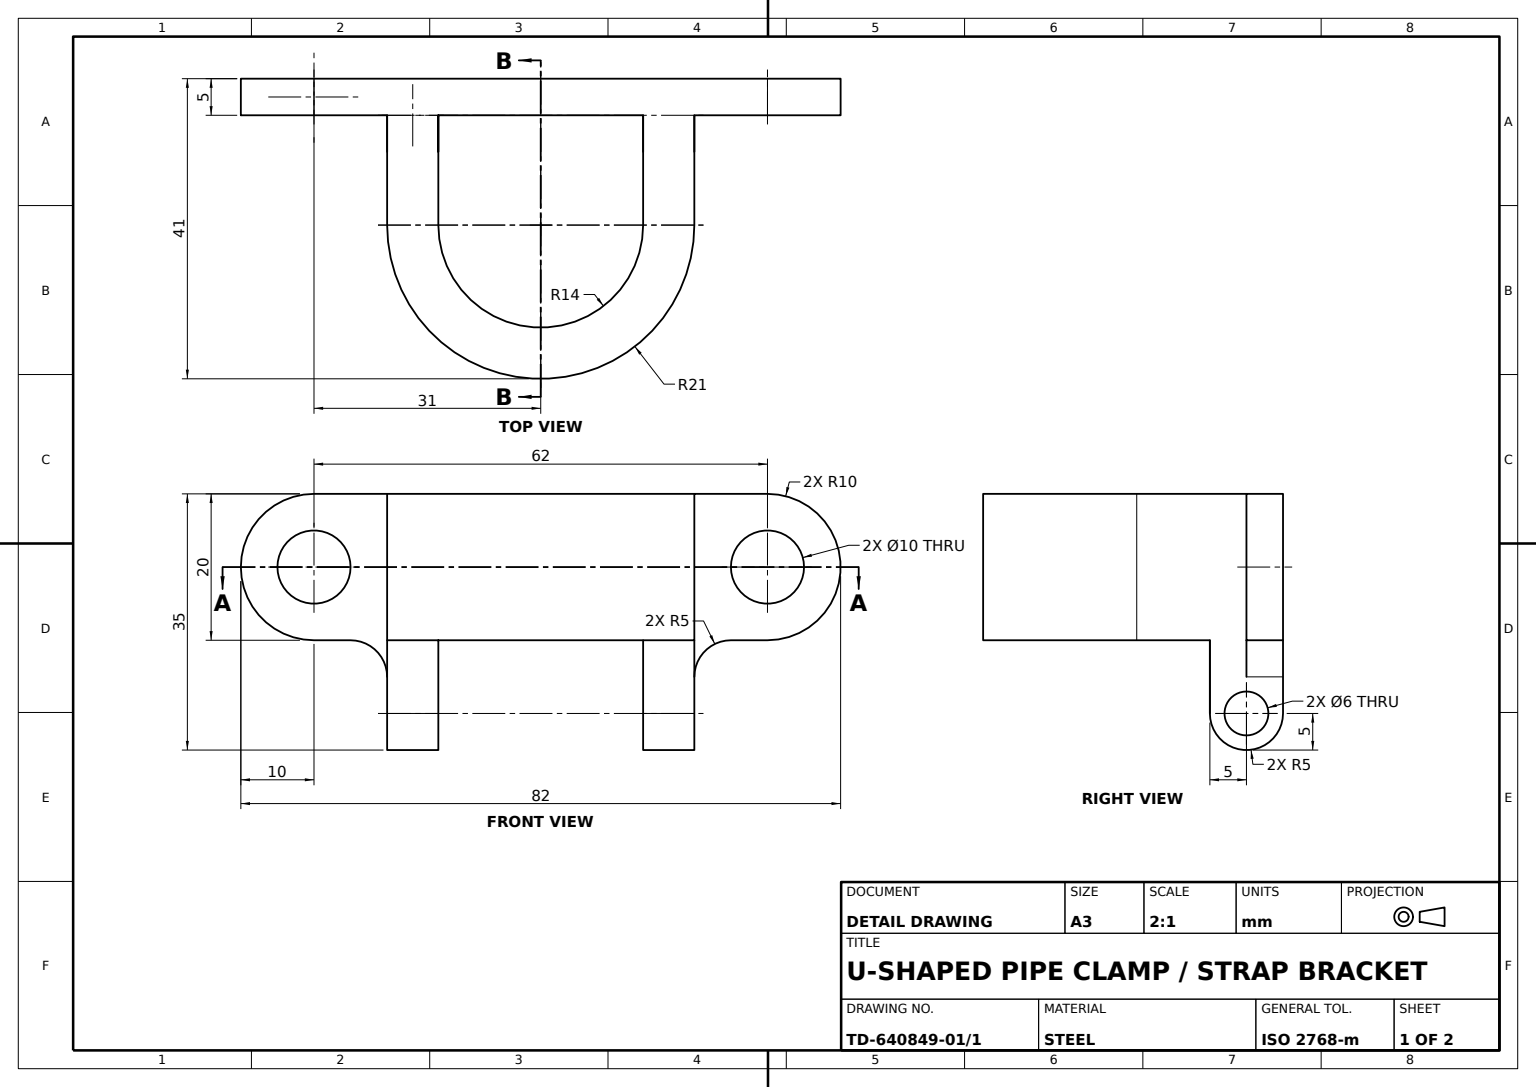
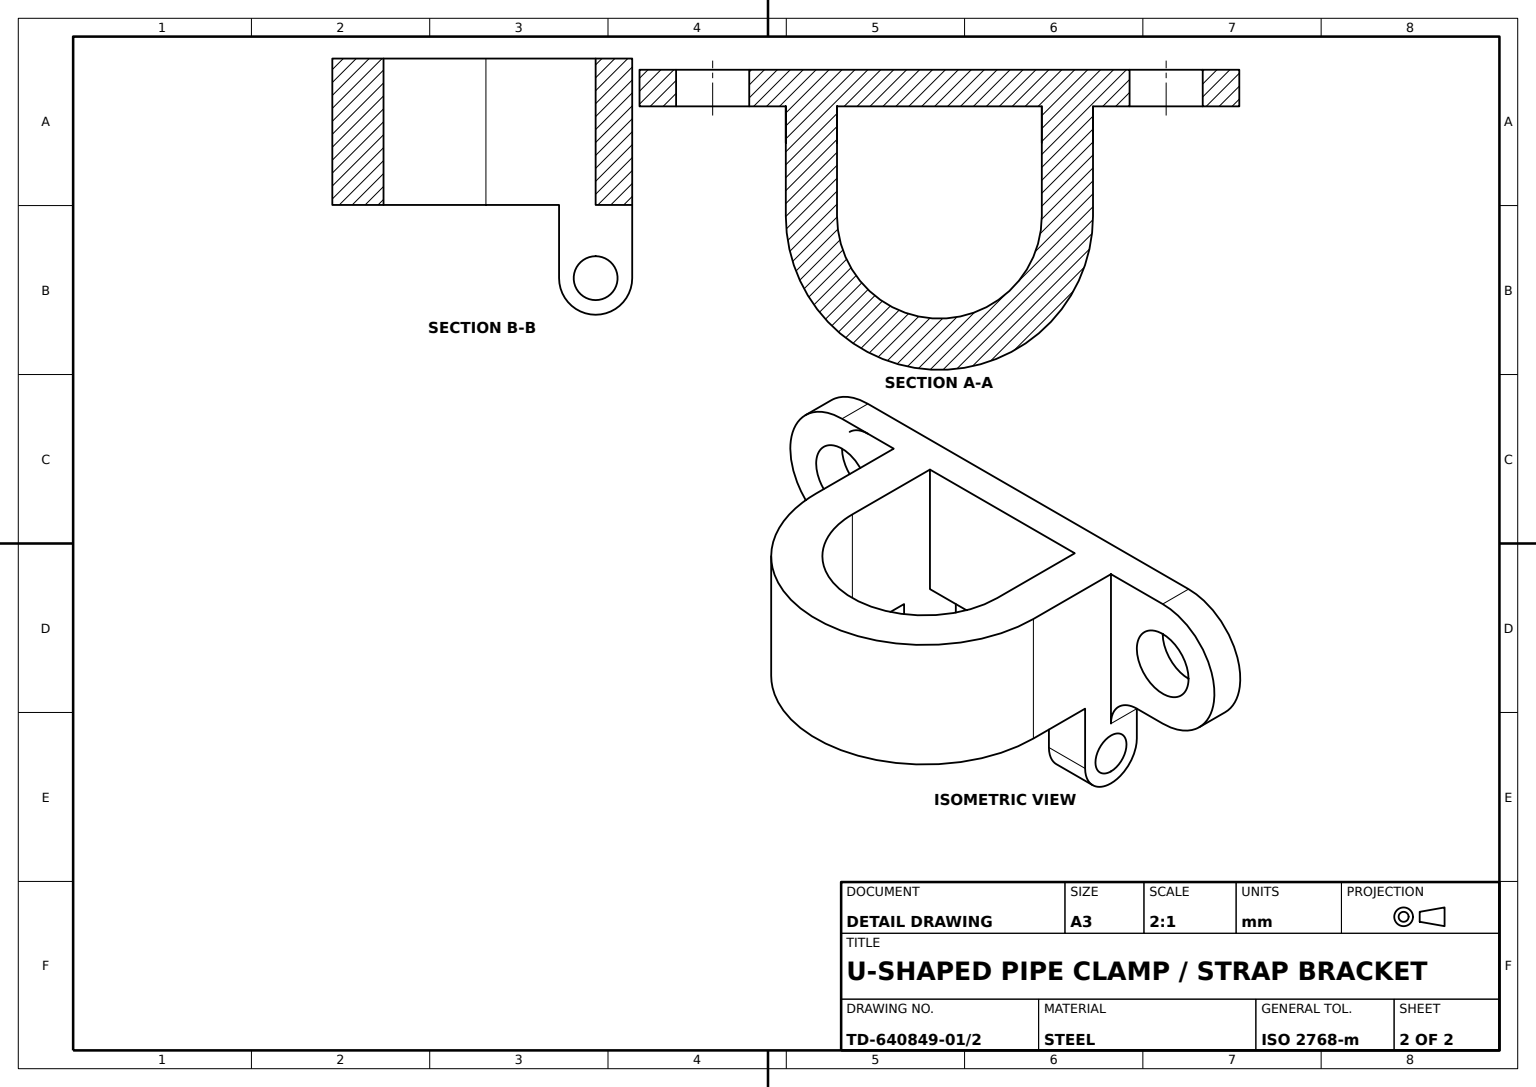
SolidWorks part; units mm, degrees
material "Plain Carbon Steel"
ref_plane "Front Plane" through (0, 0, 0) normal (0, 0, 1) x (1, 0, 0)
ref_plane "Top Plane" through (0, 0, 0) normal (0, 1, 0) x (1, 0, 0)
ref_plane "Right Plane" through (0, 0, 0) normal (1, 0, 0) x (0, 0, -1)
sketch "Base Flange Sketch" plane through (0, 0, 0) normal (0, 0, 1) x (1, 0, 0)
  line L2 (0, 10) -> (62, 10)
  line L4 (62, -10) -> (0, -10)
  line L5 (0, -10) -> (10, -10)
  arc A0 (0, 10) -> (0, -10) centre (0, 0) ccw
  arc A1 (62, -10) -> (62, 10) centre (62, 0) ccw
  dimension "D1" = 20
  dimension "D2" = 20
  dimension "D3" = 10
  dimension "D4" = 52
  dimension "D5" = 62
extrude "Base Flange" add sketch "Base Flange Sketch" along normal blind 5 contours L4 A1 L2 A0
sketch "Clamp Body Sketch" plane through (0, -10, 0) normal (0, -1, 0) x (1, 0, 0)
  line L0 (10, 5) -> (52, 5)
  line L1 (62, 5) -> (0, 5) construction
  line L2 (10, 5) -> (10, 20)
  line L3 (62, 5) -> (62, 0) construction
  line L4 (52, 5) -> (52, 20)
  line L5 (62, 0) -> (0, 0) construction
  arc A0 (52, 20) -> (10, 20) centre (31, 20) ccw
  dimension "D1" = 42
  dimension "D2" = 21
  dimension "D3" = 31
  dimension "D4" = 20
extrude "Clamp Body" add sketch "Clamp Body Sketch" against normal blind 20
sketch "Bore Sketch" plane through (0, -10, 0) normal (0, -1, 0) x (1, 0, 0)
  line L1 (17, 5) -> (17, 20)
  line L3 (45, 5) -> (45, 20)
  line L4 (17, 5) -> (45, 5)
  arc A0 (45, 20) -> (17, 20) centre (31, 20) ccw
  dimension "D1" = 28
  dimension "D2" = 28
  dimension "D3" = 15
  dimension "D4" = 31
  dimension "D5" = 20
extrude "Bore Ø28" cut sketch "Bore Sketch" against normal blind 20
sketch "Flange Cut Sketch" plane through (0, 0, 5) normal (0, 0, 1) x (1, 0, 0)
  circle A0 centre (62, 0) radius 5
  circle A1 centre (0, 0) radius 5
  dimension "D1" = 10
  dimension "D2" = 10
  dimension "D3" = 10
extrude "Flange Cut" cut sketch "Flange Cut Sketch" against normal blind 20
sketch "Lug A Sketch" plane through (0, 0, 5) normal (0, 0, 1) x (1, 0, 0)
  line L0 (10, -10) -> (5, -10)
  line L1 (17, -20) -> (17, -10)
  line L2 (10, -15) -> (10, -20)
  line L3 (10, -20) -> (17, -20)
  line L4 (17, -10) -> (10, -10)
  line L5 (10, 10) -> (10, -10) construction
  arc A0 (10, -15) -> (5, -10) centre (5, -15) ccw
  dimension "D1" = 10
  dimension "D2" = 5
  dimension "D3" = 7
extrude "Lug A" add sketch "Lug A Sketch" against normal blind 5
sketch "Lug A Web Sketch" plane through (17, 0, 0) normal (1, 0, 0) x (0, 0, -1)
  line L0 (-5, -20) -> (-10, -20)
  line L1 (-10, -20) -> (-10, -10)
  line L2 (-5, -10) -> (-20, -10) construction
  line L3 (-10, -10) -> (-5, -10)
  line L4 (-5, -10) -> (-5, -20)
  line L5 (-5, -20) -> (-5, -10) construction
  dimension "D1" = 5
extrude "Lug A Web" add sketch "Lug A Web Sketch" against normal blind 7
sketch "Lug B Sketch" plane through (0, 0, 5) normal (0, 0, 1) x (1, 0, 0)
  line L0 (52, -10) -> (57, -10)
  line L1 (52, -20) -> (45, -20)
  line L2 (62, -10) -> (52, -10) construction
  line L4 (52, -15) -> (52, -20)
  line L5 (45, -20) -> (45, -10)
  line L6 (45, -10) -> (52, -10)
  arc A0 (57, -10) -> (52, -15) centre (57, -15) ccw
  dimension "D1" = 10
extrude "Lug B" add sketch "Lug B Sketch" against normal blind 5
sketch "Lug Bridge Sketch" plane through (45, 0, 0) normal (-1, 0, 0) x (0, 0, 1)
  line L0 (10, -10) -> (10, -20)
  line L1 (10, -20) -> (5, -20)
  line L2 (0, -20) -> (10, -20) construction
  line L3 (5, -20) -> (5, -10)
  line L4 (5, -10) -> (10, -10)
extrude "Lug Bridge" add sketch "Lug Bridge Sketch" against normal blind 7
sketch "Ear A Sketch" plane through (10, 0, 0) normal (-1, 0, 0) x (0, 0, 1)
  line L0 (0, -20) -> (10, -20) construction
  line L1 (0, -20) -> (10, -20)
  arc A0 (0, -20) -> (10, -20) centre (5, -20) ccw
  dimension "D1" = 10
extrude "Ear A" add sketch "Ear A Sketch" against normal blind 7
sketch "Ear B Sketch" plane through (52, 0, 0) normal (1, 0, 0) x (0, 0, -1)
  line L0 (0, -20) -> (-10, -20) construction
  line L1 (-10, -20) -> (0, -20)
  arc A0 (-10, -20) -> (0, -20) centre (-5, -20) ccw
  dimension "D1" = 10
extrude "Ear B" add sketch "Ear B Sketch" against normal blind 7
sketch "Clamp Bolt Hole Sketch" plane through (52, 0, 0) normal (1, 0, 0) x (0, 0, -1)
  circle A0 centre (-5, -20) radius 3
  dimension "D1" = 6
  dimension "D2" = 6
extrude "Clamp Bolt Hole Ø6" cut sketch "Clamp Bolt Hole Sketch" against normal blind 70
